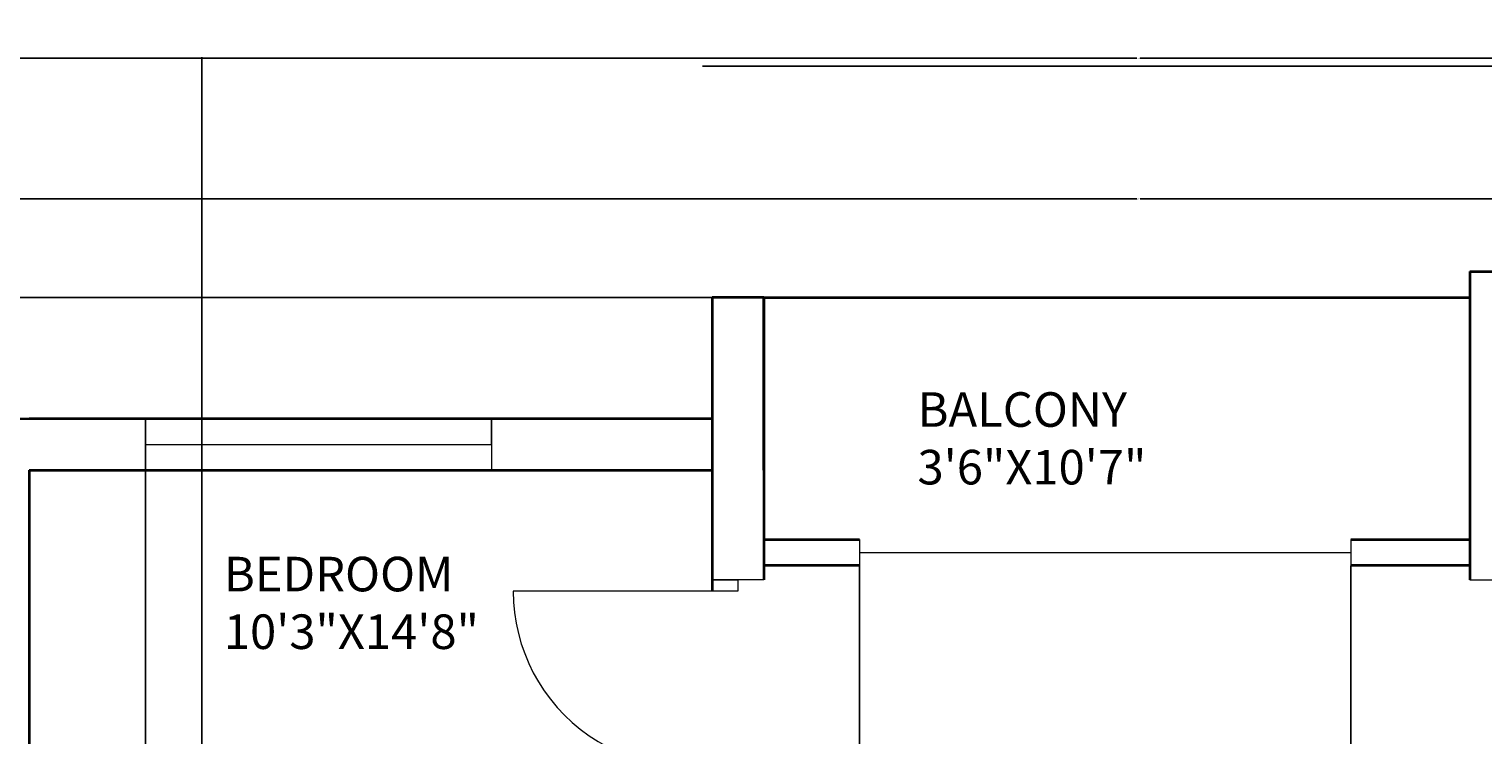
# Model space of a CAD drawing. Units: inches. Extents: x 1854 to 2495, y 1460 to 2772.
# Tile 10 of 12: x 1987 to 2239, y 2192 to 2314. Entities that reach past the tile are written whole.
import ezdxf

# ---------------------------------------------------------------- set-up
doc = ezdxf.new("R2010")
doc.units = ezdxf.units.IN
for name, color, linetype, lineweight in [('A-ANNO-DIMS', 2, 'Continuous', 18), ('A-ANNO-TEXT', 7, 'Continuous', 25), ('A-AREA-IDEN', 7, 'Continuous', 18), ('A-DOOR', 3, 'Continuous', 18), ('A-GLAZ', 4, 'Continuous', 18), ('A-WALL', 7, 'Continuous', 35)]:
    doc.layers.add(name, color=color, linetype=linetype, lineweight=lineweight)
doc.styles.get("Standard").update_dxf_attribs({"font": 'arial.ttf'})
doc.dimstyles.get("Standard").update_dxf_attribs({"dimtxt": 0.18, "dimasz": 0.18, "dimexe": 0.18, "dimexo": 0.0625, "dimgap": 0.09, "dimtad": 0, "dimtih": 1, "dimtoh": 1, "dimdec": 4, "dimzin": 0, "dimdsep": 46, "dimtxsty": 'Standard', "dimcen": 0.09, "dimadec": 0, "dimazin": 0, "dimtfac": 1, "dimtdec": 4, "dimtofl": 0, "dimtmove": 0, "dimatfit": 3, "dimfxl": 1, "dimtolj": 1, "dimtzin": 0, "dimarcsym": 0})

# ---------------------------------------------------------------- blocks, each defined once
blk = doc.blocks.new('WINDOW-60IN')
for p, q in [((0, 9), (0, 0)), ((60, 4.5), (60, 9)), ((60, 9), (60, 0)), ((0, 0), (0, 4.5)), ((0, 4.5), (60, 4.5))]:
    blk.add_line(p, q)
blk = doc.blocks.new('*D49')
at = {"layer": 'A-ANNO-DIMS', "color": 0, "lineweight": -2, "transparency": 16777216}
for p, q in [((1977.98, 2246.51), (1977.98, 2309.27)), ((1978.16, 2309.09), (2179.19, 2309.09)), ((2380.8, 2309.09), (2179.77, 2309.09)), ((2380.98, 2272.11), (2380.98, 2309.27))]:
    blk.add_line(p, q, dxfattribs=at)
at = {"layer": 'A-ANNO-DIMS', "color": 0, "transparency": 16777216}
for points in [[(1978.16, 2309.12), (1978.16, 2309.06), (1977.98, 2309.09)], [(2380.8, 2309.12), (2380.8, 2309.06), (2380.98, 2309.09)]]:
    blk.add_solid(points, dxfattribs=at)
at = {"layer": 'Defpoints', "color": 0, "transparency": 16777216}
for p in [(2380.98, 2309.09), (2380.98, 2272.04), (1977.98, 2246.45)]:
    blk.add_point(p, dxfattribs=at)
at = {"layer": 'A-ANNO-DIMS', "color": 0, "transparency": 16777216, "insert": (2179.48, 2309.09), "char_height": 0.18, "attachment_point": 5}
blk.add_mtext('\\A1;403', dxfattribs=at)
blk = doc.blocks.new('*D50')
at = {"layer": 'A-ANNO-DIMS', "color": 0, "lineweight": -2, "transparency": 16777216}
for p, q in [((2381.04, 2272.04), (2418.21, 2272.04)), ((2418.03, 2271.86), (2418.03, 1933.48)), ((2418.03, 1594.72), (2418.03, 1933.11)), ((2119.04, 1594.54), (2418.21, 1594.54))]:
    blk.add_line(p, q, dxfattribs=at)
at = {"layer": 'A-ANNO-DIMS', "color": 0, "transparency": 16777216}
for points in [[(2418, 2271.86), (2418.06, 2271.86), (2418.03, 2272.04)], [(2418, 1594.72), (2418.06, 1594.72), (2418.03, 1594.54)]]:
    blk.add_solid(points, dxfattribs=at)
at = {"layer": 'Defpoints', "color": 0, "transparency": 16777216}
for p in [(2380.98, 2272.04), (2418.03, 2272.04), (2118.98, 1594.54)]:
    blk.add_point(p, dxfattribs=at)
at = {"layer": 'A-ANNO-DIMS', "color": 0, "transparency": 16777216, "insert": (2418.03, 1933.29), "char_height": 0.18, "attachment_point": 5}
blk.add_mtext('\\A1;677.5', dxfattribs=at)
blk = doc.blocks.new('*D57')
at = {"layer": 'A-ANNO-DIMS', "color": 0, "lineweight": -2, "transparency": 16777216}
for p, q in [((2105.42, 2267.54), (1940.75, 2267.54)), ((1940.93, 2267.36), (1940.93, 2257.18)), ((1940.93, 2246.63), (1940.93, 2256.82)), ((1977.92, 2246.45), (1940.75, 2246.45))]:
    blk.add_line(p, q, dxfattribs=at)
at = {"layer": 'A-ANNO-DIMS', "color": 0, "transparency": 16777216}
for points in [[(1940.9, 2267.36), (1940.96, 2267.36), (1940.93, 2267.54)], [(1940.9, 2246.63), (1940.96, 2246.63), (1940.93, 2246.45)]]:
    blk.add_solid(points, dxfattribs=at)
at = {"layer": 'Defpoints', "color": 0, "transparency": 16777216}
for p in [(1940.93, 2267.54), (2105.48, 2267.54), (1977.98, 2246.45)]:
    blk.add_point(p, dxfattribs=at)
at = {"layer": 'A-ANNO-DIMS', "color": 0, "transparency": 16777216, "insert": (1940.93, 2257), "char_height": 0.18, "attachment_point": 5}
blk.add_mtext('\\A1;21.095', dxfattribs=at)
blk = doc.blocks.new('*D61')
at = {"layer": 'A-ANNO-DIMS', "color": 0, "lineweight": -2, "transparency": 16777216}
for p, q in [((1977.98, 1847.11), (1977.98, 2309.27)), ((1978.16, 2309.09), (1997.26, 2309.09)), ((2016.8, 2309.09), (1997.7, 2309.09)), ((2016.98, 1847.11), (2016.98, 2309.27))]:
    blk.add_line(p, q, dxfattribs=at)
at = {"layer": 'A-ANNO-DIMS', "color": 0, "transparency": 16777216}
for points in [[(1978.16, 2309.12), (1978.16, 2309.06), (1977.98, 2309.09)], [(2016.8, 2309.12), (2016.8, 2309.06), (2016.98, 2309.09)]]:
    blk.add_solid(points, dxfattribs=at)
at = {"layer": 'Defpoints', "color": 0, "transparency": 16777216}
for p in [(2016.98, 2309.09), (1977.98, 1847.04), (2016.98, 1847.04)]:
    blk.add_point(p, dxfattribs=at)
at = {"layer": 'A-ANNO-DIMS', "color": 0, "transparency": 16777216, "insert": (1997.48, 2309.09), "char_height": 0.18, "attachment_point": 5}
blk.add_mtext('\\A1;39', dxfattribs=at)
blk = doc.blocks.new('*D63')
at = {"layer": 'A-ANNO-DIMS', "color": 0, "lineweight": -2, "transparency": 16777216}
for p, q in [((1977.98, 2246.39), (1977.98, 1503.44)), ((2007.19, 2246.48), (2007.19, 1503.44)), ((1978.16, 1503.62), (1992.21, 1503.62)), ((2007.01, 1503.62), (1992.96, 1503.62))]:
    blk.add_line(p, q, dxfattribs=at)
at = {"layer": 'A-ANNO-DIMS', "color": 0, "transparency": 16777216}
for points in [[(1978.16, 1503.65), (1978.16, 1503.59), (1977.98, 1503.62)], [(2007.01, 1503.65), (2007.01, 1503.59), (2007.19, 1503.62)]]:
    blk.add_solid(points, dxfattribs=at)
at = {"layer": 'Defpoints', "color": 0, "transparency": 16777216}
for p in [(1977.98, 2246.45), (2007.19, 2246.54), (2007.19, 1503.62)]:
    blk.add_point(p, dxfattribs=at)
at = {"layer": 'A-ANNO-DIMS', "color": 0, "transparency": 16777216, "insert": (1992.59, 1503.62), "char_height": 0.18, "attachment_point": 5}
blk.add_mtext('\\A1;29.21', dxfattribs=at)
blk = doc.blocks.new('*D73')
at = {"layer": 'A-ANNO-DIMS', "color": 0, "lineweight": -2, "transparency": 16777216}
for p, q in [((2131.08, 2220.98), (2131.08, 1503.44)), ((2216.32, 2220.98), (2216.32, 1503.44)), ((2131.26, 1503.62), (2173.31, 1503.62)), ((2216.14, 1503.62), (2174.1, 1503.62))]:
    blk.add_line(p, q, dxfattribs=at)
at = {"layer": 'A-ANNO-DIMS', "color": 0, "transparency": 16777216}
for points in [[(2131.26, 1503.65), (2131.26, 1503.59), (2131.08, 1503.62)], [(2216.14, 1503.65), (2216.14, 1503.59), (2216.32, 1503.62)]]:
    blk.add_solid(points, dxfattribs=at)
at = {"layer": 'Defpoints', "color": 0, "transparency": 16777216}
for p in [(2131.08, 2221.04), (2216.32, 2221.04), (2216.32, 1503.62)]:
    blk.add_point(p, dxfattribs=at)
at = {"layer": 'A-ANNO-DIMS', "color": 0, "transparency": 16777216, "insert": (2173.7, 1503.62), "char_height": 0.18, "attachment_point": 5}
blk.add_mtext('\\A1;85.25', dxfattribs=at)
blk = doc.blocks.new('*D74')
at = {"layer": 'A-ANNO-DIMS', "color": 0, "lineweight": -2, "transparency": 16777216}
for p, q in [((1953.98, 2372.03), (1953.98, 2284.46)), ((2404.98, 2372.03), (2404.98, 2284.46)), ((1954.16, 2284.64), (2179.21, 2284.64)), ((2404.8, 2284.64), (2179.76, 2284.64))]:
    blk.add_line(p, q, dxfattribs=at)
at = {"layer": 'A-ANNO-DIMS', "color": 0, "transparency": 16777216}
for points in [[(1954.16, 2284.67), (1954.16, 2284.61), (1953.98, 2284.64)], [(2404.8, 2284.67), (2404.8, 2284.61), (2404.98, 2284.64)]]:
    blk.add_solid(points, dxfattribs=at)
at = {"layer": 'Defpoints', "color": 0, "transparency": 16777216}
for p in [(1953.98, 2372.09), (2404.98, 2372.09), (2404.98, 2284.64)]:
    blk.add_point(p, dxfattribs=at)
at = {"layer": 'A-ANNO-DIMS', "color": 0, "transparency": 16777216, "insert": (2179.48, 2284.64), "char_height": 0.18, "attachment_point": 5}
blk.add_mtext('\\A1;451', dxfattribs=at)

msp = doc.modelspace()

# ---------------------------------------------------------------- linework, layer by layer
at = {"layer": 'A-ANNO-TEXT'}
msp.add_line((2103.8101, 2307.6905), (2254.3702, 2307.6905), dxfattribs=at)
at = {"layer": 'A-DOOR'}
for p, q in [((2114.4824, 2218.5567), (2105.4824, 2218.5567)), ((2105.4824, 2218.5567), (2109.9824, 2218.5567)), ((2109.9824, 2218.5567), (2109.9824, 2216.5567)), ((2109.9824, 2218.5567), (2109.9824, 2218.5567)), ((2109.9824, 2218.5567), (2109.9824, 2216.5567)), ((2236.9824, 2218.5567), (2245.9824, 2218.5567)), ((2073.9824, 2216.5567), (2070.9824, 2216.5567)), ((2109.9824, 2216.5567), (2073.9824, 2216.5567))]:
    msp.add_line(p, q, dxfattribs=at)
msp.add_arc((2101.4541, 2216.5567), 30.4717, 180, 290.714797, dxfattribs=at)
at = {"layer": 'A-GLAZ'}
for p, q in [((2067.1898, 2246.5449), (2067.1898, 2246.5449)), ((2131.0775, 2225.5449), (2131.0775, 2221.0449)), ((2216.3239, 2225.5449), (2216.3239, 2221.0449)), ((2131.0775, 2223.2949), (2216.3239, 2223.2949))]:
    msp.add_line(p, q, dxfattribs=at)
at = {"layer": 'A-WALL'}
for p, q in [((2236.9824, 2272.0449), (2236.9824, 2218.5567)), ((2236.9824, 2272.0449), (2380.9824, 2272.0449)), ((2114.4824, 2267.5449), (2105.4824, 2267.5449)), ((2105.4824, 2267.5449), (2105.4824, 2216.5567)), ((2114.4824, 2264.5449), (2114.4824, 2267.5449)), ((2114.4824, 2267.5449), (2236.9824, 2267.5449)), ((2114.4824, 2267.5449), (2114.4824, 2225.5449)), ((2114.4824, 2246.5449), (2114.4824, 2264.5449)), ((1977.9824, 2246.45), (1986.9824, 2246.5449)), ((1986.9824, 2246.5449), (2105.4824, 2246.5449)), ((2114.4824, 2237.5449), (2114.4824, 2246.5449)), ((1986.9824, 2237.5449), (1986.9824, 2070.5449)), ((1986.9824, 2237.5449), (2105.4824, 2237.5449)), ((2114.4824, 2237.5449), (2114.4824, 2218.5567)), ((2114.4824, 2225.5449), (2131.0775, 2225.5449)), ((2216.3239, 2225.5449), (2236.9824, 2225.5449)), ((2236.9824, 2225.5449), (2236.9824, 2221.0449)), ((2131.0775, 2221.0449), (2114.4824, 2221.0449)), ((2236.9824, 2221.0449), (2216.3239, 2221.0449))]:
    msp.add_line(p, q, dxfattribs=at)

# ---------------------------------------------------------------- block references
at = {"layer": 'A-GLAZ'}
msp.add_blockref('WINDOW-60IN', (2007.19, 2237.545), dxfattribs=at)

# ---------------------------------------------------------------- texts
at = {"layer": 'A-AREA-IDEN', "char_height": 6, "attachment_point": 1}
for s, width, insert in [('BALCONY\\P3\'6"X10\'7"', 102.145105, (2141.1279, 2251.0944)), ('BEDROOM\\P10\'3"X14\'8"', 102.999072, (2020.7761, 2222.5353))]:
    msp.add_mtext_dynamic_manual_height_columns(s, width=width, gutter_width=12.5, heights=[0], dxfattribs=dict(at, insert=insert))

# ---------------------------------------------------------------- dimensions: what is measured, and where the dimension line sits
at = {"layer": 'A-ANNO-DIMS'}
for base, p1, p2, override, picture, middle in [((2404.9824, 2284.6405), (1953.9824, 2372.0884), (2404.9824, 2372.0884), {"dimdec": 0, "dimlfac": 1, "dimrnd": 0, "dimzin": 0, "dimdsep": 46, "dimlunit": 2}, '*D74', (2179.4824, 2284.6405)), ((2380.9824, 2309.0949), (1977.9824, 2246.45), (2380.9824, 2272.0449), {"dimdec": 0, "dimlfac": 1, "dimrnd": 0, "dimzin": 0, "dimdsep": 46, "dimlunit": 2}, '*D49', (2179.4824, 2309.0949)), ((2016.9824, 2309.0949), (1977.9824, 1847.0449), (2016.9824, 1847.0449), {"dimdec": 0, "dimlfac": 1, "dimrnd": 0, "dimzin": 0, "dimdsep": 46, "dimlunit": 2}, '*D61', (1997.4824, 2309.0949)), ((2007.1898, 1503.6207), (1977.9824, 2246.45), (2007.1898, 2246.5449), {"dimdec": 2, "dimlfac": 1, "dimrnd": 0, "dimzin": 0, "dimdsep": 46, "dimlunit": 2}, '*D63', (1992.5861, 1503.6207)), ((2216.3239, 1503.6207), (2131.0775, 2221.0449), (2216.3239, 2221.0449), {"dimdec": 2, "dimlfac": 1, "dimrnd": 0, "dimzin": 0, "dimdsep": 46, "dimlunit": 2}, '*D73', (2173.7007, 1503.6207))]:
    dim = msp.add_linear_dim(base=base, p1=p1, p2=p2, dimstyle='Standard', override=override, dxfattribs=at)
    dim.commit()
    dim.dimension.update_dxf_attribs({"geometry": picture, "text_midpoint": middle})
for base, p1, p2, override, picture, middle in [((2418.0324, 2272.0449), (2118.9824, 1594.5449), (2380.9824, 2272.0449), {"dimdec": 1, "dimlfac": 1, "dimrnd": 0, "dimzin": 0, "dimdsep": 46, "dimlunit": 2}, '*D50', (2418.0324, 1933.2949)), ((1940.9324, 2267.5449), (1977.9824, 2246.45), (2105.4824, 2267.5449), {"dimdec": 3, "dimlfac": 1, "dimrnd": 0, "dimzin": 0, "dimdsep": 46, "dimlunit": 2}, '*D57', (1940.9324, 2256.9975))]:
    dim = msp.add_linear_dim(base=base, p1=p1, p2=p2, angle=90, dimstyle='Standard', override=override, dxfattribs=at)
    dim.commit()
    dim.dimension.update_dxf_attribs({"geometry": picture, "text_midpoint": middle})

doc.saveas('drawing.dxf')
